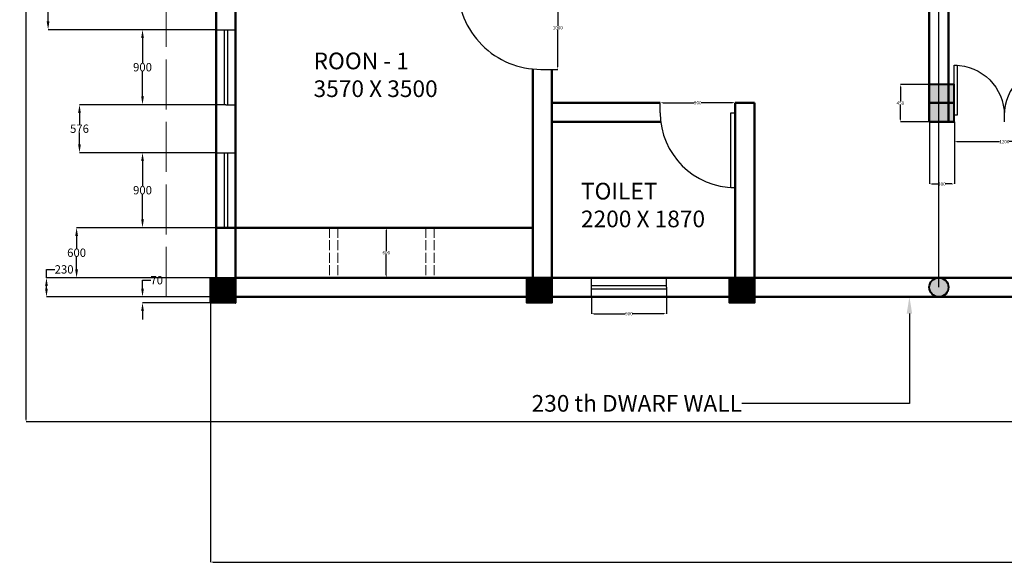
# Model space of a CAD drawing. Units: millimetres. Extents: x -17156 to 39375, y -45872 to -24892.
# Tile 1 of 12: x -17156 to -5337, y -45872 to -39337. Entities that reach past the tile are written whole.
import ezdxf
from ezdxf import colors
from ezdxf.entities.mleader import LeaderData, LeaderLine
from ezdxf.math import Vec2, Vec3

# ---------------------------------------------------------------- set-up
doc = ezdxf.new("R2010")
doc.units = ezdxf.units.MM
doc.header["$MEASUREMENT"] = 0
doc.linetypes.add('ACAD_ISO02W100', pattern=[15, 12, -3])
for name, color, linetype, lineweight in [('A-ANNO-DIMS', 2, 'Continuous', 18), ('A-ANNO-TEXT', 4, 'Continuous', 18), ('A-AREA-IDEN', 4, 'Continuous', 25), ('A-COLS', 7, 'Continuous', 40), ('A-FLOR-FIXT-HIDN', 8, 'ACAD_ISO02W100', 18), ('A-ROOF-OVHD', 8, 'ACAD_ISO02W100', 18), ('DOORS', 6, 'Continuous', 25), ('WALLS', 5, 'Continuous', 50), ('WINDOW', 240, 'Continuous', 25)]:
    doc.layers.add(name, color=color, linetype=linetype, lineweight=lineweight)
doc.layers.add('A-COLS-PATT', color=114, linetype='Continuous', lineweight=13, true_color=0x139b48)
doc.styles.get("Standard").update_dxf_attribs({"font": 'arial.ttf'})
doc.dimstyles.get("Standard").update_dxf_attribs({"dimtxt": 40, "dimasz": 30.18, "dimexe": 0, "dimexo": 0.0625, "dimgap": 0.09, "dimtad": 0, "dimtih": 1, "dimtoh": 1, "dimdec": 0, "dimzin": 0, "dimdsep": 46, "dimtxsty": 'Standard', "dimcen": 0.09, "dimadec": 0, "dimazin": 0, "dimtfac": 1, "dimtdec": 0, "dimtofl": 0, "dimtmove": 0, "dimatfit": 3, "dimfxl": 1, "dimtolj": 1, "dimtzin": 0, "dimarcsym": 0})

# ---------------------------------------------------------------- blocks, each defined once
blk = doc.blocks.new('*U6')
for p, q in [((-750, 0), (-750, 100)), ((0, 0), (0, 100))]:
    blk.add_line(p, q)
blk.add_lwpolyline([(0, 0), (0, -750), (-43.75, -750), (-43.75, 0)], close=True)
blk.add_arc((0, 0), 750, 180, 270)
blk = doc.blocks.new('*U7')
for p, q in [((0, 0), (0, 100)), ((750, 0), (750, 100))]:
    blk.add_line(p, q)
blk.add_lwpolyline([(0, 0), (0, -750), (43.75, -750), (43.75, 0)], close=True)
blk.add_arc((0, 0), 750, 270, 0)
blk = doc.blocks.new('*D9')
at = {"layer": 'A-ANNO-DIMS', "color": 0, "lineweight": -2, "transparency": 16777216}
for p, q in [((-15682, -42563), (-15682, -42463)), ((-15682, -42463), (-15582, -42463)), ((-14797, -42663), (-15682, -42663)), ((-14867, -42733), (-15682, -42733)), ((-15682, -42833), (-15682, -42933))]:
    blk.add_line(p, q, dxfattribs=at)
at = {"layer": 'A-ANNO-DIMS', "color": 0, "lineweight": 100, "transparency": 16777216}
for points in [[(-15698, -42563), (-15665, -42563), (-15682, -42663)], [(-15698, -42833), (-15665, -42833), (-15682, -42733)]]:
    blk.add_solid(points, dxfattribs=at)
at = {"layer": 'Defpoints', "color": 0, "lineweight": 100, "transparency": 16777216}
for p in [(-15682, -42663), (-14797, -42663), (-14867, -42733)]:
    blk.add_point(p, dxfattribs=at)
at = {"layer": 'A-ANNO-DIMS', "color": 0, "transparency": 16777216, "insert": (-15511, -42463), "char_height": 100, "attachment_point": 5}
blk.add_mtext('\\A1;70', dxfattribs=at)
blk = doc.blocks.new('*D10')
at = {"layer": 'A-ANNO-DIMS', "color": 0, "lineweight": -2, "transparency": 16777216}
for p, q in [((-16835, -42433), (-16835, -42333)), ((-16835, -42333), (-16735, -42333)), ((-14867, -42433), (-16835, -42433)), ((-16835, -42563), (-16835, -42533)), ((-14797, -42663), (-16835, -42663))]:
    blk.add_line(p, q, dxfattribs=at)
at = {"layer": 'A-ANNO-DIMS', "color": 0, "lineweight": 100, "transparency": 16777216}
for points in [[(-16851, -42533), (-16818, -42533), (-16835, -42433)], [(-16851, -42563), (-16818, -42563), (-16835, -42663)]]:
    blk.add_solid(points, dxfattribs=at)
at = {"layer": 'Defpoints', "color": 0, "lineweight": 100, "transparency": 16777216}
for p in [(-16835, -42433), (-14867, -42433), (-14797, -42663)]:
    blk.add_point(p, dxfattribs=at)
at = {"layer": 'A-ANNO-DIMS', "color": 0, "transparency": 16777216, "insert": (-16623, -42333), "char_height": 100, "attachment_point": 5}
blk.add_mtext('\\A1;230', dxfattribs=at)
blk = doc.blocks.new('*D11')
at = {"layer": 'A-ANNO-DIMS', "color": 0, "lineweight": -2, "transparency": 16777216}
for p, q in [((-14797, -41833), (-16473, -41833)), ((-16473, -41933), (-16473, -42082)), ((-16473, -42333), (-16473, -42184)), ((-14867, -42433), (-16473, -42433))]:
    blk.add_line(p, q, dxfattribs=at)
at = {"layer": 'A-ANNO-DIMS', "color": 0, "lineweight": 100, "transparency": 16777216}
for points in [[(-16490, -41933), (-16456, -41933), (-16473, -41833)], [(-16490, -42333), (-16456, -42333), (-16473, -42433)]]:
    blk.add_solid(points, dxfattribs=at)
at = {"layer": 'Defpoints', "color": 0, "lineweight": 100, "transparency": 16777216}
for p in [(-16473, -41833), (-14797, -41833), (-14867, -42433)]:
    blk.add_point(p, dxfattribs=at)
at = {"layer": 'A-ANNO-DIMS', "color": 0, "transparency": 16777216, "insert": (-16473, -42133), "char_height": 100, "attachment_point": 5}
blk.add_mtext('\\A1;600', dxfattribs=at)
blk = doc.blocks.new('*D12')
at = {"layer": 'A-ANNO-DIMS', "color": 0, "lineweight": -2, "transparency": 16777216}
for p, q in [((-14797, -40933), (-15682, -40933)), ((-15682, -41033), (-15682, -41332)), ((-15682, -41733), (-15682, -41434)), ((-14797, -41833), (-15682, -41833))]:
    blk.add_line(p, q, dxfattribs=at)
at = {"layer": 'A-ANNO-DIMS', "color": 0, "lineweight": 100, "transparency": 16777216}
for points in [[(-15698, -41033), (-15665, -41033), (-15682, -40933)], [(-15698, -41733), (-15665, -41733), (-15682, -41833)]]:
    blk.add_solid(points, dxfattribs=at)
at = {"layer": 'Defpoints', "color": 0, "lineweight": 100, "transparency": 16777216}
for p in [(-15682, -40933), (-14797, -40933), (-14797, -41833)]:
    blk.add_point(p, dxfattribs=at)
at = {"layer": 'A-ANNO-DIMS', "color": 0, "transparency": 16777216, "insert": (-15682, -41383), "char_height": 100, "attachment_point": 5}
blk.add_mtext('\\A1;900', dxfattribs=at)
blk = doc.blocks.new('*D13')
at = {"layer": 'A-ANNO-DIMS', "color": 0, "lineweight": -2, "transparency": 16777216}
for p, q in [((-14797, -40357), (-16438, -40357)), ((-16438, -40457), (-16438, -40594)), ((-16438, -40833), (-16438, -40696)), ((-14797, -40933), (-16438, -40933))]:
    blk.add_line(p, q, dxfattribs=at)
at = {"layer": 'A-ANNO-DIMS', "color": 0, "lineweight": 100, "transparency": 16777216}
for points in [[(-16455, -40457), (-16422, -40457), (-16438, -40357)], [(-16455, -40833), (-16422, -40833), (-16438, -40933)]]:
    blk.add_solid(points, dxfattribs=at)
at = {"layer": 'Defpoints', "color": 0, "lineweight": 100, "transparency": 16777216}
for p in [(-16438, -40357), (-14797, -40357), (-14797, -40933)]:
    blk.add_point(p, dxfattribs=at)
at = {"layer": 'A-ANNO-DIMS', "color": 0, "transparency": 16777216, "insert": (-16438, -40645), "char_height": 100, "attachment_point": 5}
blk.add_mtext('\\A1;576', dxfattribs=at)
blk = doc.blocks.new('*D14')
at = {"layer": 'A-ANNO-DIMS', "color": 0, "lineweight": -2, "transparency": 16777216}
for p, q in [((-14797, -39457), (-15682, -39457)), ((-15682, -39557), (-15682, -39856)), ((-15682, -40257), (-15682, -39958)), ((-14797, -40357), (-15682, -40357))]:
    blk.add_line(p, q, dxfattribs=at)
at = {"layer": 'A-ANNO-DIMS', "color": 0, "lineweight": 100, "transparency": 16777216}
for points in [[(-15698, -39557), (-15665, -39557), (-15682, -39457)], [(-15698, -40257), (-15665, -40257), (-15682, -40357)]]:
    blk.add_solid(points, dxfattribs=at)
at = {"layer": 'Defpoints', "color": 0, "lineweight": 100, "transparency": 16777216}
for p in [(-15682, -39457), (-14797, -39457), (-14797, -40357)]:
    blk.add_point(p, dxfattribs=at)
at = {"layer": 'A-ANNO-DIMS', "color": 0, "transparency": 16777216, "insert": (-15682, -39907), "char_height": 100, "attachment_point": 5}
blk.add_mtext('\\A1;900', dxfattribs=at)
blk = doc.blocks.new('*D15')
at = {"layer": 'A-ANNO-DIMS', "color": 0, "lineweight": -2, "transparency": 16777216}
for p, q in [((-16815, -39003), (-16815, -38803)), ((-16815, -38803), (-16715, -38803)), ((-14867, -39003), (-16815, -39003)), ((-16815, -39357), (-16815, -39103)), ((-14797, -39457), (-16815, -39457))]:
    blk.add_line(p, q, dxfattribs=at)
at = {"layer": 'A-ANNO-DIMS', "color": 0, "lineweight": 100, "transparency": 16777216}
for points in [[(-16832, -39103), (-16799, -39103), (-16815, -39003)], [(-16832, -39357), (-16799, -39357), (-16815, -39457)]]:
    blk.add_solid(points, dxfattribs=at)
at = {"layer": 'Defpoints', "color": 0, "lineweight": 100, "transparency": 16777216}
for p in [(-16815, -39003), (-14867, -39003), (-14797, -39457)]:
    blk.add_point(p, dxfattribs=at)
at = {"layer": 'A-ANNO-DIMS', "color": 0, "transparency": 16777216, "insert": (-16603, -38803), "char_height": 100, "attachment_point": 5}
blk.add_mtext('\\A1;454', dxfattribs=at)
blk = doc.blocks.new('*D88')
at = {"layer": 'A-ANNO-DIMS', "color": 0, "lineweight": -2, "transparency": 16777216}
for p, q in [((-12897, -41833), (-12756, -41833)), ((-12756, -41863), (-12756, -42112)), ((-12756, -42403), (-12756, -42153)), ((-12965, -42433), (-12756, -42433))]:
    blk.add_line(p, q, dxfattribs=at)
at = {"layer": 'A-ANNO-DIMS', "color": 0, "lineweight": 100, "transparency": 16777216}
for points in [[(-12761, -41863), (-12751, -41863), (-12756, -41833)], [(-12761, -42403), (-12751, -42403), (-12756, -42433)]]:
    blk.add_solid(points, dxfattribs=at)
at = {"layer": 'Defpoints', "color": 0, "lineweight": 100, "transparency": 16777216}
for p in [(-12897, -41833), (-12756, -41833), (-12965, -42433)]:
    blk.add_point(p, dxfattribs=at)
at = {"layer": 'A-ANNO-DIMS', "color": 0, "transparency": 16777216, "insert": (-12756, -42133), "char_height": 40, "attachment_point": 5}
blk.add_mtext('\\A1;600', dxfattribs=at)
blk = doc.blocks.new('*D89')
at = {"layer": 'A-ANNO-DIMS', "color": 0, "lineweight": -2, "transparency": 16777216}
for p, q in [((-10697, -38933), (-10697, -38933)), ((-10697, -38963), (-10697, -39412)), ((-10697, -39903), (-10697, -39453)), ((-10767, -39933), (-10697, -39933))]:
    blk.add_line(p, q, dxfattribs=at)
at = {"layer": 'A-ANNO-DIMS', "color": 0, "lineweight": 100, "transparency": 16777216}
for points in [[(-10702, -38963), (-10692, -38963), (-10697, -38933)], [(-10702, -39903), (-10692, -39903), (-10697, -39933)]]:
    blk.add_solid(points, dxfattribs=at)
at = {"layer": 'Defpoints', "color": 0, "lineweight": 100, "transparency": 16777216}
for p in [(-10697, -38933), (-10697, -38933), (-10767, -39933)]:
    blk.add_point(p, dxfattribs=at)
at = {"layer": 'A-ANNO-DIMS', "color": 0, "transparency": 16777216, "insert": (-10697, -39433), "char_height": 40, "attachment_point": 5}
blk.add_mtext('\\A1;1000', dxfattribs=at)
blk = doc.blocks.new('*D90')
at = {"layer": 'A-ANNO-DIMS', "color": 0, "lineweight": -2, "transparency": 16777216}
for p, q in [((-9467, -40333), (-9467, -40333)), ((-9437, -40333), (-9062, -40333)), ((-8598, -40333), (-8973, -40333)), ((-8567, -40333), (-8567, -40333))]:
    blk.add_line(p, q, dxfattribs=at)
at = {"layer": 'A-ANNO-DIMS', "color": 0, "lineweight": 100, "transparency": 16777216}
for points in [[(-9437, -40328), (-9437, -40338), (-9467, -40333)], [(-8598, -40328), (-8598, -40338), (-8567, -40333)]]:
    blk.add_solid(points, dxfattribs=at)
at = {"layer": 'Defpoints', "color": 0, "lineweight": 100, "transparency": 16777216}
for p in [(-9467, -40333), (-8567, -40333), (-8567, -40333)]:
    blk.add_point(p, dxfattribs=at)
at = {"layer": 'A-ANNO-DIMS', "color": 0, "transparency": 16777216, "insert": (-9017, -40333), "char_height": 40, "attachment_point": 5}
blk.add_mtext('\\A1;900', dxfattribs=at)
blk = doc.blocks.new('*D91')
at = {"layer": 'A-ANNO-DIMS', "color": 0, "lineweight": -2, "transparency": 16777216}
for p, q in [((-10293, -42663), (-10293, -42865)), ((-9393, -42663), (-9393, -42865)), ((-10263, -42865), (-9888, -42865)), ((-9424, -42865), (-9799, -42865))]:
    blk.add_line(p, q, dxfattribs=at)
at = {"layer": 'A-ANNO-DIMS', "color": 0, "lineweight": 100, "transparency": 16777216}
for points in [[(-10263, -42860), (-10263, -42871), (-10293, -42865)], [(-9424, -42860), (-9424, -42871), (-9393, -42865)]]:
    blk.add_solid(points, dxfattribs=at)
at = {"layer": 'Defpoints', "color": 0, "lineweight": 100, "transparency": 16777216}
for p in [(-10293, -42663), (-9393, -42663), (-9393, -42865)]:
    blk.add_point(p, dxfattribs=at)
at = {"layer": 'A-ANNO-DIMS', "color": 0, "transparency": 16777216, "insert": (-9843, -42865), "char_height": 40, "attachment_point": 5}
blk.add_mtext('\\A1;900', dxfattribs=at)
blk = doc.blocks.new('*D92')
at = {"layer": 'A-ANNO-DIMS', "color": 0, "lineweight": -2, "transparency": 16777216}
for p, q in [((-6237, -40113), (-6584, -40113)), ((-6584, -40143), (-6584, -40317)), ((-6584, -40533), (-6584, -40358)), ((-6237, -40563), (-6584, -40563))]:
    blk.add_line(p, q, dxfattribs=at)
at = {"layer": 'A-ANNO-DIMS', "color": 0, "lineweight": 100, "transparency": 16777216}
for points in [[(-6589, -40143), (-6579, -40143), (-6584, -40113)], [(-6589, -40533), (-6579, -40533), (-6584, -40563)]]:
    blk.add_solid(points, dxfattribs=at)
at = {"layer": 'Defpoints', "color": 0, "lineweight": 100, "transparency": 16777216}
for p in [(-6237, -40113), (-6584, -40563), (-6237, -40563)]:
    blk.add_point(p, dxfattribs=at)
at = {"layer": 'A-ANNO-DIMS', "color": 0, "transparency": 16777216, "insert": (-6584, -40338), "char_height": 40, "attachment_point": 5}
blk.add_mtext('\\A1;450', dxfattribs=at)
blk = doc.blocks.new('*D93')
at = {"layer": 'A-ANNO-DIMS', "color": 0, "lineweight": -2, "transparency": 16777216}
for p, q in [((-6237, -40563), (-6237, -41308)), ((-5937, -40563), (-5937, -41308)), ((-6207, -41308), (-6132, -41308)), ((-5968, -41308), (-6043, -41308))]:
    blk.add_line(p, q, dxfattribs=at)
at = {"layer": 'A-ANNO-DIMS', "color": 0, "lineweight": 100, "transparency": 16777216}
for points in [[(-6207, -41303), (-6207, -41313), (-6237, -41308)], [(-5968, -41303), (-5968, -41313), (-5937, -41308)]]:
    blk.add_solid(points, dxfattribs=at)
at = {"layer": 'Defpoints', "color": 0, "lineweight": 100, "transparency": 16777216}
for p in [(-6237, -40563), (-5937, -40563), (-5937, -41308)]:
    blk.add_point(p, dxfattribs=at)
at = {"layer": 'A-ANNO-DIMS', "color": 0, "transparency": 16777216, "insert": (-6087, -41308), "char_height": 40, "attachment_point": 5}
blk.add_mtext('\\A1;300', dxfattribs=at)
blk = doc.blocks.new('*D94')
at = {"layer": 'A-ANNO-DIMS', "color": 0, "lineweight": -2, "transparency": 16777216}
for p, q in [((-5937, -40563), (-5937, -40800)), ((-4737, -40563), (-4737, -40800)), ((-5907, -40800), (-5395, -40800)), ((-4768, -40800), (-5279, -40800))]:
    blk.add_line(p, q, dxfattribs=at)
at = {"layer": 'A-ANNO-DIMS', "color": 0, "lineweight": 100, "transparency": 16777216}
for points in [[(-5907, -40795), (-5907, -40805), (-5937, -40800)], [(-4768, -40795), (-4768, -40805), (-4737, -40800)]]:
    blk.add_solid(points, dxfattribs=at)
at = {"layer": 'Defpoints', "color": 0, "lineweight": 100, "transparency": 16777216}
for p in [(-5937, -40563), (-4737, -40563), (-5937, -40800)]:
    blk.add_point(p, dxfattribs=at)
at = {"layer": 'A-ANNO-DIMS', "color": 0, "transparency": 16777216, "insert": (-5337, -40800), "char_height": 40, "attachment_point": 5}
blk.add_mtext('\\A1;1200', dxfattribs=at)
blk = doc.blocks.new('WIN-900x230')
for p, q in [((0, 900), (230, 900)), ((95, 900), (95, 0)), ((135, 900), (135, 0)), ((115, 0), (0, 0)), ((115, 0), (230, 0))]:
    blk.add_line(p, q)
blk = doc.blocks.new('COL-300x300')
h = blk.add_hatch()
h.set_pattern_fill('ANSI31', color=256)
h.paths.add_polyline_path([(300, 300), (0, 300), (0, 0), (300, 0)])
blk.add_lwpolyline([(0, 300), (300, 300), (300, 0), (0, 0)], close=True)
blk = doc.blocks.new('COL-450x300')
h = blk.add_hatch(color=256)
h.dxf.hatch_style = 1
h.paths.add_polyline_path([(0, 300), (0, 0), (450, 0), (450, 300)])
blk.add_lwpolyline([(0, 300), (0, 0), (450, 0), (450, 300)], close=True)
blk = doc.blocks.new('*D145')
at = {"layer": 'A-ANNO-DIMS', "color": 0, "lineweight": -2, "transparency": 16777216}
for p, q in [((-6237, -27248), (-17080, -27248)), ((-17080, -27278), (-17080, -35685)), ((-17080, -44133), (-17080, -35726)), ((-2887, -44163), (-17080, -44163))]:
    blk.add_line(p, q, dxfattribs=at)
at = {"layer": 'A-ANNO-DIMS', "color": 0, "lineweight": 100, "transparency": 16777216}
for points in [[(-17085, -27278), (-17075, -27278), (-17080, -27248)], [(-17085, -44133), (-17075, -44133), (-17080, -44163)]]:
    blk.add_solid(points, dxfattribs=at)
at = {"layer": 'Defpoints', "color": 0, "lineweight": 100, "transparency": 16777216}
for p in [(-6237, -27248), (-17080, -44163), (-2887, -44163)]:
    blk.add_point(p, dxfattribs=at)
at = {"layer": 'A-ANNO-DIMS', "color": 0, "transparency": 16777216, "insert": (-17080, -35705), "char_height": 40, "attachment_point": 5}
blk.add_mtext('\\A1;16915', dxfattribs=at)
blk = doc.blocks.new('*D146')
at = {"layer": 'A-ANNO-DIMS', "color": 0, "lineweight": -2, "transparency": 16777216}
for p, q in [((-14867, -42733), (-14867, -45846)), ((13043, -42733), (13043, -45846)), ((-14837, -45846), (-988, -45846)), ((13012, -45846), (-837, -45846))]:
    blk.add_line(p, q, dxfattribs=at)
at = {"layer": 'A-ANNO-DIMS', "color": 0, "lineweight": 100, "transparency": 16777216}
for points in [[(-14837, -45841), (-14837, -45851), (-14867, -45846)], [(13012, -45841), (13012, -45851), (13043, -45846)]]:
    blk.add_solid(points, dxfattribs=at)
at = {"layer": 'Defpoints', "color": 0, "lineweight": 100, "transparency": 16777216}
for p in [(-14867, -42733), (13043, -42733), (13043, -45846)]:
    blk.add_point(p, dxfattribs=at)
at = {"layer": 'A-ANNO-DIMS', "color": 0, "transparency": 16777216, "insert": (-912, -45846), "char_height": 40, "attachment_point": 5}
blk.add_mtext('\\A1;27910', dxfattribs=at)
blk = doc.blocks.new('*D151')
at = {"layer": 'A-ANNO-DIMS', "color": 0, "lineweight": -2, "transparency": 16777216}
for p, q in [((-6122, -42548), (-6122, -25565)), ((-6092, -25565), (-4413, -25565)), ((-2615, -25565), (-4294, -25565)), ((-2584, -42548), (-2584, -25565))]:
    blk.add_line(p, q, dxfattribs=at)
at = {"layer": 'A-ANNO-DIMS', "color": 0, "lineweight": 100, "transparency": 16777216}
for points in [[(-6092, -25560), (-6092, -25570), (-6122, -25565)], [(-2615, -25560), (-2615, -25570), (-2584, -25565)]]:
    blk.add_solid(points, dxfattribs=at)
at = {"layer": 'Defpoints', "color": 0, "lineweight": 100, "transparency": 16777216}
for p in [(-2584, -25565), (-6122, -42548), (-2584, -42548)]:
    blk.add_point(p, dxfattribs=at)
at = {"layer": 'A-ANNO-DIMS', "color": 0, "transparency": 16777216, "insert": (-4353, -25565), "char_height": 40, "attachment_point": 5}
blk.add_mtext('\\A1;3538', dxfattribs=at)

msp = doc.modelspace()

# ---------------------------------------------------------------- hatches: boundary and pattern name
at = {"layer": 'A-COLS-PATT'}
h = msp.add_hatch(color=256, dxfattribs=at)
h.dxf.hatch_style = 1
h.paths.add_polyline_path([(-6007.35, -42547.85, 1), (-6237.35, -42547.85, 1)])
h.paths.add_polyline_path([(-2699.35, -42547.85, 1), (-2469.35, -42547.85, 1)])
h.paths.add_polyline_path([(424.65, -42547.85, 1), (654.65, -42547.85, 1)])
h.paths.add_polyline_path([(3997.65, -42547.85, 1), (4227.65, -42547.85, 1)])
h.paths.add_polyline_path([(1581.84, -34499.85), (1481.84, -34499.85), (1481.84, -34599.85), (1581.84, -34599.85)])
h.paths.add_polyline_path([(3181.84, -34499.85), (3081.84, -34499.85), (3081.84, -34599.85), (3181.84, -34599.85)])
h.paths.add_polyline_path([(-162.32, -34499.85), (-262.32, -34499.85), (-262.32, -34599.85), (-162.32, -34599.85)])
h.paths.add_polyline_path([(-1762.32, -34499.85), (-1862.32, -34499.85), (-1862.32, -34599.85), (-1762.32, -34599.85)])
h.paths.add_polyline_path([(-3445.85, -34499.85), (-3545.85, -34499.85), (-3545.85, -34599.85), (-3445.85, -34599.85)])
h.paths.add_polyline_path([(-5045.85, -34499.85), (-5145.85, -34499.85), (-5145.85, -34599.85), (-5045.85, -34599.85)])

# ---------------------------------------------------------------- linework, layer by layer
at = {"layer": 'A-COLS'}
msp.add_circle((-6122.35, -42547.85), 115, dxfattribs=at)
at = {"layer": 'A-FLOR-FIXT-HIDN', "ltscale": 10}
for p, q in [((-13438.8, -41832.85), (-13438.8, -42432.85)), ((-13338.8, -41832.85), (-13338.8, -42432.85)), ((-12282.58, -41832.85), (-12282.58, -42432.85)), ((-12182.58, -41832.85), (-12182.58, -42432.85))]:
    msp.add_line(p, q, dxfattribs=at)
at = {"layer": 'A-ROOF-OVHD', "ltscale": 50}
msp.add_line((-15397.35, -42662.85), (-15397.35, -31007.85), dxfattribs=at)
at = {"layer": 'WALLS'}
for p, q in [((-6007.35, -27247.85), (-6007.35, -40562.85)), ((-14797.35, -42662.85), (-14797.35, -31607.85)), ((-6237.35, -33152.85), (-6237.35, -40562.85)), ((-14567.35, -42432.85), (-14567.35, -38932.85)), ((-10997.35, -42662.85), (-10997.35, -39928.16)), ((-10767.35, -42662.85), (-10767.35, -39932.85)), ((-9467.35, -40332.85), (-10767.35, -40332.85)), ((-8567.35, -42662.85), (-8567.35, -40332.85)), ((-8337.35, -40332.85), (-8567.35, -40332.85)), ((-8337.35, -42662.85), (-8337.35, -40332.85)), ((-6237.35, -40332.85), (-5937.35, -40332.85)), ((-9460.6, -40562.85), (-10767.35, -40562.85)), ((-6237.35, -40562.85), (-5937.35, -40562.85)), ((-10997.35, -41832.85), (-14797.35, -41832.85)), ((-10997.35, -42432.85), (-14567.35, -42432.85)), ((12592.65, -42432.85), (-10997.35, -42432.85)), ((12822.65, -42662.85), (-14797.35, -42662.85))]:
    msp.add_line(p, q, dxfattribs=at)

# ---------------------------------------------------------------- block references
at = {"layer": 'A-COLS', "rotation": 90.00000000000138}
msp.add_blockref('COL-450x300', (-5937.35, -40562.85), dxfattribs=at)
at = {"layer": 'A-COLS'}
for p in [(-14867.35, -42732.85), (-11067.35, -42732.85), (-8637.35, -42732.85)]:
    msp.add_blockref('COL-300x300', p, dxfattribs=at)
at = {"layer": 'DOORS'}
for p, xscale, yscale, zscale, rotation in [((-10900.68, -38932.85), 1.333333333333333, 1.333333333333333, 1.333333333333333, 270), ((-5937.35, -40482.85), -0.8, 0.8, 0.8, 180), ((-4737.35, -40482.85), 0.8, 0.8, 0.8, 180)]:
    msp.add_blockref('*U7', p, dxfattribs=dict(at, xscale=xscale, yscale=yscale, zscale=zscale, rotation=rotation))
at = {"layer": 'DOORS', "xscale": 1.199999999999999, "yscale": 1.199999999999999, "zscale": 1.199999999999999}
msp.add_blockref('*U6', (-8567.35, -40452.85), dxfattribs=at)
at = {"layer": 'WINDOW'}
for p in [(-14797.35, -40356.9), (-14797.35, -41832.85)]:
    msp.add_blockref('WIN-900x230', p, dxfattribs=at)
at = {"layer": 'WINDOW', "rotation": 90.00000000000017}
msp.add_blockref('WIN-900x230', (-9393.36, -42662.85), dxfattribs=at)

# ---------------------------------------------------------------- texts
at = {"layer": 'A-AREA-IDEN', "char_height": 200, "attachment_point": 1}
for s, width, insert in [('{ROON - 1\\P3570 X 3500}', 1724.2288, (-13628.88, -39731.52)), ('{TOILET\\P2200 X 1870}', 2176.4856, (-10419.12, -41294.18))]:
    msp.add_mtext_dynamic_manual_height_columns(s, width=width, gutter_width=1, heights=[0], dxfattribs=dict(at, insert=insert))

# ---------------------------------------------------------------- dimensions: what is measured, and where the dimension line sits
at = {"layer": 'A-ANNO-DIMS'}
for base, p1, p2, override, picture, middle in [((-2584.35, -25564.85), (-6122.35, -42547.85), (-2584.35, -42547.85), {"dimdec": 0, "dimlfac": 1, "dimrnd": 0, "dimzin": 0, "dimdsep": 46, "dimlunit": 2}, '*D151', (-4353.35, -25564.85)), ((-8567.35, -40332.85), (-9467.35, -40332.85), (-8567.35, -40332.85), {"dimclrd": 0, "dimclre": 0, "dimclrt": 0}, '*D90', (-9017.35, -40332.85)), ((-5937.35, -41307.66), (-6237.35, -40562.85), (-5937.35, -40562.85), {"dimclrd": 0, "dimclre": 0, "dimclrt": 0}, '*D93', (-6087.35, -41307.66)), ((-5937.35, -40799.77), (-4737.35, -40562.85), (-5937.35, -40562.85), {"dimclrd": 0, "dimclre": 0, "dimclrt": 0}, '*D94', (-5337.35, -40799.77)), ((-9393.36, -42865.49), (-10293.36, -42662.85), (-9393.36, -42662.85), {"dimclrd": 0, "dimclre": 0, "dimclrt": 0}, '*D91', (-9843.36, -42865.49)), ((13042.65, -45845.85), (-14867.35, -42732.85), (13042.65, -42732.85), {"dimdec": 0, "dimlfac": 1, "dimrnd": 0, "dimzin": 0, "dimdsep": 46, "dimlunit": 2}, '*D146', (-912.35, -45845.85))]:
    dim = msp.add_linear_dim(base=base, p1=p1, p2=p2, dimstyle='Standard', override=override, dxfattribs=at)
    dim.commit()
    dim.dimension.update_dxf_attribs({"geometry": picture, "text_midpoint": middle})
for base, p1, p2, angle, override, picture, middle in [((-17080.35, -44162.85), (-6237.35, -27247.85), (-2887.35, -44162.85), 90, {"dimdec": 0, "dimlfac": 1, "dimrnd": 0, "dimzin": 0, "dimdsep": 46, "dimlunit": 2}, '*D145', (-17080.35, -35705.35)), ((-10697.36, -38932.85), (-10767.35, -39932.85), (-10697.35, -38932.85), 90, {"dimclrd": 0, "dimclre": 0, "dimclrt": 0}, '*D89', (-10697.36, -39432.85)), ((-15681.77, -39456.9), (-14797.35, -40356.9), (-14797.35, -39456.9), 270, {"dimtxt": 100, "dimasz": 100, "dimclrd": 0, "dimclre": 0, "dimclrt": 0}, '*D14', (-15681.77, -39906.9)), ((-6584.43, -40562.85), (-6237.35, -40112.85), (-6237.35, -40562.85), 90, {"dimclrd": 0, "dimclre": 0, "dimclrt": 0}, '*D92', (-6584.43, -40337.85)), ((-16438.37, -40356.9), (-14797.35, -40932.85), (-14797.35, -40356.9), 270, {"dimtxt": 100, "dimasz": 100, "dimclrd": 0, "dimclre": 0, "dimclrt": 0}, '*D13', (-16438.37, -40644.87)), ((-15681.77, -40932.85), (-14797.35, -41832.85), (-14797.35, -40932.85), 270, {"dimtxt": 100, "dimasz": 100, "dimclrd": 0, "dimclre": 0, "dimclrt": 0}, '*D12', (-15681.77, -41382.85)), ((-16473.16, -41832.85), (-14867.35, -42432.85), (-14797.35, -41832.85), 270, {"dimtxt": 100, "dimasz": 100, "dimclrd": 0, "dimclre": 0, "dimclrt": 0}, '*D11', (-16473.16, -42132.85)), ((-12755.96, -41832.85), (-12964.65, -42432.85), (-12897.35, -41832.85), 90, {"dimclrd": 0, "dimclre": 0, "dimclrt": 0}, '*D88', (-12755.96, -42132.85)), ((-16834.57, -42432.85), (-14797.35, -42662.85), (-14867.35, -42432.85), 270, {"dimtxt": 100, "dimasz": 100, "dimclrd": 0, "dimclre": 0, "dimclrt": 0}, '*D10', (-16623.33, -42332.85)), ((-15681.77, -42662.85), (-14867.35, -42732.85), (-14797.35, -42662.85), 270, {"dimtxt": 100, "dimasz": 100, "dimclrd": 0, "dimclre": 0, "dimclrt": 0}, '*D9', (-15510.64, -42462.85))]:
    dim = msp.add_linear_dim(base=base, p1=p1, p2=p2, angle=angle, dimstyle='Standard', override=override, dxfattribs=at)
    dim.commit()
    dim.dimension.update_dxf_attribs({"geometry": picture, "text_midpoint": middle})
dim = msp.add_linear_dim(base=(-16815.49, -39002.85), p1=(-14797.35, -39456.9), p2=(-14867.35, -39002.85), angle=270, dimstyle='Standard', override={"dimtxt": 100, "dimasz": 100, "dimclrd": 0, "dimclre": 0, "dimclrt": 0}, dxfattribs=at)
dim.commit()
dim.dimension.update_dxf_attribs({"geometry": '*D15', "text_midpoint": (-16603.12, -38802.85), "dimtype": 160})

# ---------------------------------------------------------------- leaders
at = {"layer": 'A-ANNO-TEXT'}
ml = msp.add_multileader_mtext('Standard', dxfattribs=at)
ml.set_content('{\\C4;230 th DWARF WALL}', color=256)
ml.set_leader_properties()
ml.build(insert=Vec2(0, 0))
ml.multileader.update_dxf_attribs({"dogleg_length": 0.36, "arrow_head_size": 200})
ctx = ml.context
ctx.base_point, ctx.char_height, ctx.arrow_head_size, ctx.landing_gap_size, ctx.plane_origin = Vec3(-11185.87, -43942.43), 200, 200, 0.09, Vec3(-6476.3, -42662.85)
ctx.text_align_type = 2
notes = []
notes.append((ctx, [(0, (1, 1, 0), (-8486.28, -43942.43), (-1, 0), 0.36, [(0, [(-6476.3, -42662.85), (-6476.3, -43942.43)], 0, [])])]))
ctx.mtext.insert, ctx.mtext.alignment, ctx.mtext.flow_direction = Vec3(-8486.73, -43840.66), 3, 5
for ctx, leaders in notes:
    for number, flags, end, landing, length, lines in leaders:
        leader = LeaderData()
        leader.index, (leader.has_last_leader_line, leader.has_dogleg_vector, leader.attachment_direction) = number, flags
        leader.last_leader_point, leader.dogleg_vector, leader.dogleg_length = Vec3(end), Vec3(landing), length
        for number, points, colour, breaks in lines:
            line = LeaderLine()
            line.index, line.vertices, line.color, line.breaks = number, Vec3.list(points), colors.encode_raw_color(colour), breaks
            leader.lines.append(line)
        ctx.leaders.append(leader)

doc.saveas('drawing.dxf')
